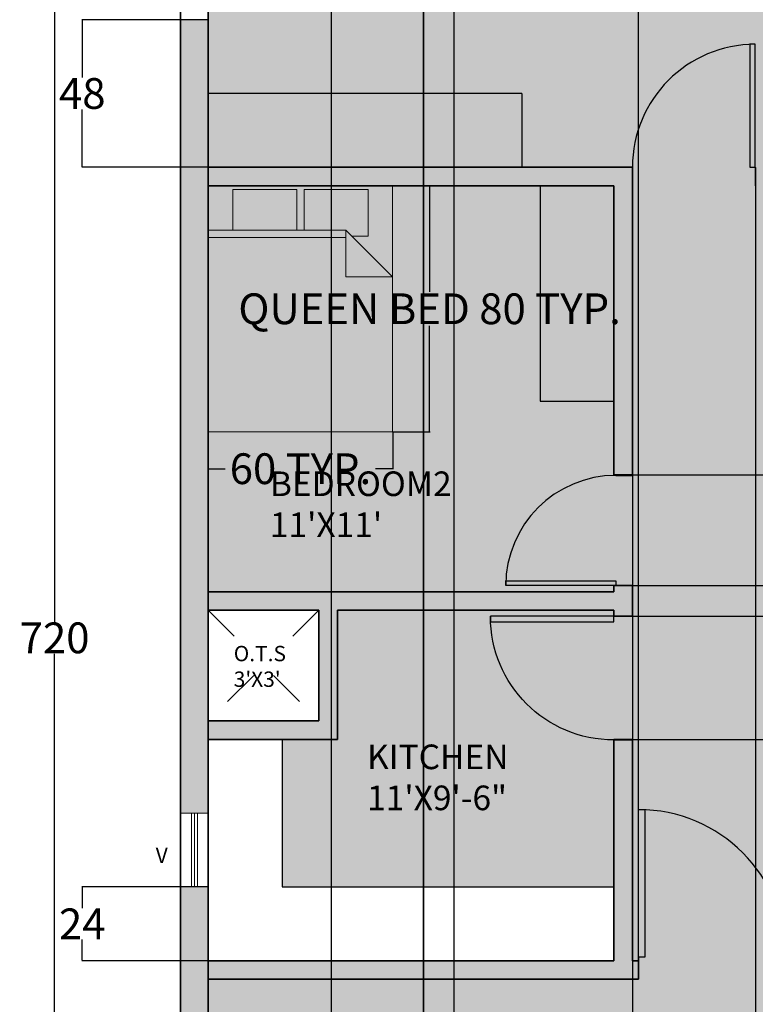
# Model space of a CAD drawing. Units: inches. Extents: x 286 to 756, y 360 to 1175.
# Tile 2 of 4: x 286 to 525, y 649 to 969. Entities that reach past the tile are written whole.
import ezdxf

# ---------------------------------------------------------------- set-up
doc = ezdxf.new("R2010")
doc.units = ezdxf.units.IN
doc.header["$MEASUREMENT"] = 0
doc.linetypes.add('ACAD_ISO03W100', pattern=[30, 12, -18])
for name, color, linetype, lineweight in [('A-ANNO-DIMS', 2, 'Continuous', 18), ('A-ANNO-TEXT', 7, 'Continuous', 18), ('A-AREA-IDEN', 7, 'Continuous', 18), ('A-FLOR-CASE', 8, 'Continuous', 25), ('A-FLOR-OPEN', 8, 'ACAD_ISO03W100', 13), ('A-GLAZ', 4, 'Continuous', 18), ('A-WALL', 7, 'Continuous', 35), ('DOOR', 6, 'Continuous', 25), ('FUR', 8, 'Continuous', 18)]:
    doc.layers.add(name, color=color, linetype=linetype, lineweight=lineweight)
for name, color, linetype, lineweight, true_color in [('A-FLOR-CASE-PATT', 30, 'Continuous', 13, 0xf8991e), ('A-FLOR-PATT', 9, 'Continuous', 13, 0xc7c8ca), ('A-WALL-PATT', 18, 'Continuous', 13, 0x000000)]:
    doc.layers.add(name, color=color, linetype=linetype, lineweight=lineweight, true_color=true_color)
doc.styles.get("Standard").update_dxf_attribs({"font": 'arial.ttf'})
doc.dimstyles.get("Standard").update_dxf_attribs({"dimtxt": 10, "dimasz": 0.18, "dimexe": 0.18, "dimexo": 0.0625, "dimgap": 0.09, "dimtad": 0, "dimtih": 1, "dimtoh": 1, "dimdec": 0, "dimzin": 0, "dimdsep": 46, "dimlunit": 3, "dimtxsty": 'Standard', "dimcen": 0.09, "dimadec": 0, "dimazin": 0, "dimtfac": 1, "dimtdec": 0, "dimtofl": 0, "dimtmove": 0, "dimatfit": 3, "dimfxl": 1, "dimtolj": 1, "dimtzin": 0, "dimarcsym": 0})

# ---------------------------------------------------------------- blocks, each defined once
blk = doc.blocks.new('*U7')
for p, q in [((0, 0), (0, -6)), ((-40, 0), (-40, -6))]:
    blk.add_line(p, q)
blk.add_lwpolyline([(0, 0), (0, 40), (-1.75, 40), (-1.75, 0)], close=True)
blk.add_arc((0, 0), 40, 90, 180)
blk = doc.blocks.new('Bed - Queen')
for p, q in [((0, -80.00003), (0, 0)), ((0, 0), (59.99999, 0)), ((59.99999, 0), (59.99999, -80.00003)), ((7.99999, -1.2), (28.79998, -1.2)), ((7.99999, -14.4), (7.99999, -1.2)), ((28.79998, -1.2), (28.79998, -14.4)), ((31.19999, -1.2), (51.99999, -1.2)), ((31.19999, -14.4), (31.19999, -1.2)), ((51.99999, -1.2), (51.99999, -16.4)), ((0, -14.4), (44.8, -14.4)), ((59.99999, -29.6), (44.8, -14.4)), ((44.8, -14.4), (44.8, -29.6)), ((44.8, -16.8), (0, -16.8)), ((51.99999, -16.4), (46.79936, -16.4)), ((44.8, -29.6), (59.99999, -29.6)), ((59.99999, -80.00003), (0, -80.00003))]:
    blk.add_line(p, q)
blk = doc.blocks.new('*U2')
for p, q in [((0, 0), (0, -6)), ((40, 0), (40, -6))]:
    blk.add_line(p, q)
blk.add_lwpolyline([(0, 0), (0, 40), (1.75, 40), (1.75, 0)], close=True)
blk.add_arc((0, 0), 40, 0, 90)
blk = doc.blocks.new('*U8')
for p, q in [((0, 0), (0, -6)), ((40, 0), (40, -6))]:
    blk.add_line(p, q)
blk.add_lwpolyline([(0, 0), (0, 40), (1.75, 40), (1.75, 0)], close=True)
blk.add_arc((0, 0), 40, 0, 90)
blk = doc.blocks.new('*D11')
at = {"layer": 'A-ANNO-DIMS', "color": 0, "lineweight": -2, "transparency": 16777216}
for p, q in [((406.93, 914.76), (419.05, 914.76)), ((418.87, 914.58), (418.87, 880.32)), ((418.87, 834.94), (418.87, 869.19)), ((406.93, 834.76), (419.05, 834.76))]:
    blk.add_line(p, q, dxfattribs=at)
at = {"layer": 'A-ANNO-DIMS', "color": 0, "transparency": 16777216}
for points in [[(418.84, 914.58), (418.9, 914.58), (418.87, 914.76)], [(418.84, 834.94), (418.9, 834.94), (418.87, 834.76)]]:
    blk.add_solid(points, dxfattribs=at)
at = {"layer": 'Defpoints', "color": 0, "transparency": 16777216}
for p in [(406.87, 914.76), (418.87, 914.76), (406.87, 834.76)]:
    blk.add_point(p, dxfattribs=at)
at = {"layer": 'A-ANNO-DIMS', "color": 0, "transparency": 16777216, "insert": (418.87, 874.76), "char_height": 10, "attachment_point": 5}
blk.add_mtext('\\A1;QUEEN BED 80 TYP.', dxfattribs=at)
blk = doc.blocks.new('*D12')
at = {"layer": 'A-ANNO-DIMS', "color": 0, "lineweight": -2, "transparency": 16777216}
for p, q in [((346.87, 834.69), (346.87, 822.58)), ((406.87, 834.69), (406.87, 822.58)), ((347.05, 822.76), (352.41, 822.76)), ((406.69, 822.76), (401.32, 822.76))]:
    blk.add_line(p, q, dxfattribs=at)
at = {"layer": 'A-ANNO-DIMS', "color": 0, "transparency": 16777216}
for points in [[(347.05, 822.79), (347.05, 822.73), (346.87, 822.76)], [(406.69, 822.79), (406.69, 822.73), (406.87, 822.76)]]:
    blk.add_solid(points, dxfattribs=at)
at = {"layer": 'Defpoints', "color": 0, "transparency": 16777216}
for p in [(346.87, 834.76), (406.87, 834.76), (406.87, 822.76)]:
    blk.add_point(p, dxfattribs=at)
at = {"layer": 'A-ANNO-DIMS', "color": 0, "transparency": 16777216, "insert": (376.87, 822.76), "char_height": 10, "attachment_point": 5}
blk.add_mtext('\\A1;60 TYP.', dxfattribs=at)
blk = doc.blocks.new('*D20')
at = {"layer": 'A-ANNO-DIMS', "color": 0, "lineweight": -2, "transparency": 16777216}
for p, q in [((346.8, 686.76), (305.69, 686.76)), ((305.87, 686.58), (305.87, 679.87)), ((305.87, 662.94), (305.87, 669.65)), ((346.8, 662.76), (305.69, 662.76))]:
    blk.add_line(p, q, dxfattribs=at)
at = {"layer": 'A-ANNO-DIMS', "color": 0, "transparency": 16777216}
for points in [[(305.84, 686.58), (305.9, 686.58), (305.87, 686.76)], [(305.84, 662.94), (305.9, 662.94), (305.87, 662.76)]]:
    blk.add_solid(points, dxfattribs=at)
at = {"layer": 'Defpoints', "color": 0, "transparency": 16777216}
for p in [(305.87, 686.76), (346.87, 686.76), (346.87, 662.76)]:
    blk.add_point(p, dxfattribs=at)
at = {"layer": 'A-ANNO-DIMS', "color": 0, "transparency": 16777216, "insert": (305.87, 674.76), "char_height": 10, "attachment_point": 5}
blk.add_mtext('\\A1;24', dxfattribs=at)
blk = doc.blocks.new('*D21')
at = {"layer": 'A-ANNO-DIMS', "color": 0, "lineweight": -2, "transparency": 16777216}
for p, q in [((346.8, 968.76), (305.69, 968.76)), ((305.87, 968.58), (305.87, 949.95)), ((305.87, 920.94), (305.87, 939.56)), ((346.8, 920.76), (305.69, 920.76))]:
    blk.add_line(p, q, dxfattribs=at)
at = {"layer": 'A-ANNO-DIMS', "color": 0, "transparency": 16777216}
for points in [[(305.84, 968.58), (305.9, 968.58), (305.87, 968.76)], [(305.84, 920.94), (305.9, 920.94), (305.87, 920.76)]]:
    blk.add_solid(points, dxfattribs=at)
at = {"layer": 'Defpoints', "color": 0, "transparency": 16777216}
for p in [(305.87, 968.76), (346.87, 968.76), (346.87, 920.76)]:
    blk.add_point(p, dxfattribs=at)
at = {"layer": 'A-ANNO-DIMS', "color": 0, "transparency": 16777216, "insert": (305.87, 944.76), "char_height": 10, "attachment_point": 5}
blk.add_mtext('\\A1;48', dxfattribs=at)
blk = doc.blocks.new('*D22')
at = {"layer": 'A-ANNO-DIMS', "color": 0, "lineweight": -2, "transparency": 16777216}
for p, q in [((337.8, 1127.76), (296.69, 1127.76)), ((296.87, 1127.58), (296.87, 772.95)), ((296.87, 407.94), (296.87, 762.56)), ((337.8, 407.76), (296.69, 407.76))]:
    blk.add_line(p, q, dxfattribs=at)
at = {"layer": 'A-ANNO-DIMS', "color": 0, "transparency": 16777216}
for points in [[(296.84, 1127.58), (296.9, 1127.58), (296.87, 1127.76)], [(296.84, 407.94), (296.9, 407.94), (296.87, 407.76)]]:
    blk.add_solid(points, dxfattribs=at)
at = {"layer": 'Defpoints', "color": 0, "transparency": 16777216}
for p in [(296.87, 1127.76), (337.87, 1127.76), (337.87, 407.76)]:
    blk.add_point(p, dxfattribs=at)
at = {"layer": 'A-ANNO-DIMS', "color": 0, "transparency": 16777216, "insert": (296.87, 767.76), "char_height": 10, "attachment_point": 5}
blk.add_mtext('\\A1;720', dxfattribs=at)
blk = doc.blocks.new('*D26')
at = {"layer": 'A-ANNO-DIMS', "color": 0, "lineweight": -2, "transparency": 16777216}
for p, q in [((346.87, 656.82), (346.87, 1168.94)), ((347.05, 1168.76), (406.22, 1168.76)), ((486.69, 1168.76), (427.51, 1168.76)), ((486.87, 656.82), (486.87, 1168.94))]:
    blk.add_line(p, q, dxfattribs=at)
at = {"layer": 'A-ANNO-DIMS', "color": 0, "transparency": 16777216}
for points in [[(347.05, 1168.79), (347.05, 1168.73), (346.87, 1168.76)], [(486.69, 1168.79), (486.69, 1168.73), (486.87, 1168.76)]]:
    blk.add_solid(points, dxfattribs=at)
at = {"layer": 'Defpoints', "color": 0, "transparency": 16777216}
for p in [(486.87, 1168.76), (346.87, 656.76), (486.87, 656.76)]:
    blk.add_point(p, dxfattribs=at)
at = {"layer": 'A-ANNO-DIMS', "color": 0, "transparency": 16777216, "insert": (416.87, 1168.76), "char_height": 10, "attachment_point": 5}
blk.add_mtext('\\A1;140', dxfattribs=at)
blk = doc.blocks.new('*D27')
at = {"layer": 'A-ANNO-DIMS', "color": 0, "lineweight": -2, "transparency": 16777216}
for p, q in [((486.87, 656.82), (486.87, 1168.94)), ((487.05, 1168.76), (503.4, 1168.76)), ((534.69, 1168.76), (518.33, 1168.76)), ((534.87, 656.82), (534.87, 1168.94))]:
    blk.add_line(p, q, dxfattribs=at)
at = {"layer": 'A-ANNO-DIMS', "color": 0, "transparency": 16777216}
for points in [[(487.05, 1168.79), (487.05, 1168.73), (486.87, 1168.76)], [(534.69, 1168.79), (534.69, 1168.73), (534.87, 1168.76)]]:
    blk.add_solid(points, dxfattribs=at)
at = {"layer": 'Defpoints', "color": 0, "transparency": 16777216}
for p in [(534.87, 1168.76), (486.87, 656.76), (534.87, 656.76)]:
    blk.add_point(p, dxfattribs=at)
at = {"layer": 'A-ANNO-DIMS', "color": 0, "transparency": 16777216, "insert": (510.87, 1168.76), "char_height": 10, "attachment_point": 5}
blk.add_mtext('\\A1;48', dxfattribs=at)
blk = doc.blocks.new('*D33')
at = {"layer": 'A-ANNO-DIMS', "color": 0, "lineweight": -2, "transparency": 16777216}
for p, q in [((416.87, 452.82), (416.87, 1168.94)), ((417.05, 1168.76), (426.69, 1168.76)), ((426.87, 452.82), (426.87, 1168.94)), ((426.87, 1168.76), (427.05, 1168.76))]:
    blk.add_line(p, q, dxfattribs=at)
at = {"layer": 'A-ANNO-DIMS', "color": 0, "transparency": 16777216}
for points in [[(417.05, 1168.79), (417.05, 1168.73), (416.87, 1168.76)], [(426.69, 1168.79), (426.69, 1168.73), (426.87, 1168.76)]]:
    blk.add_solid(points, dxfattribs=at)
at = {"layer": 'Defpoints', "color": 0, "transparency": 16777216}
for p in [(426.87, 1168.76), (416.87, 452.76), (426.87, 452.76)]:
    blk.add_point(p, dxfattribs=at)
at = {"layer": 'A-ANNO-DIMS', "color": 0, "transparency": 16777216, "insert": (433.81, 1168.76), "char_height": 10, "attachment_point": 5}
blk.add_mtext('\\A1;10', dxfattribs=at)
blk = doc.blocks.new('*D34')
at = {"layer": 'A-ANNO-DIMS', "color": 0, "lineweight": -2, "transparency": 16777216}
for p, q in [((346.87, 1064.69), (346.87, 366.58)), ((386.87, 1064.69), (386.87, 366.58)), ((347.05, 366.76), (359.43, 366.76)), ((386.69, 366.76), (374.3, 366.76))]:
    blk.add_line(p, q, dxfattribs=at)
at = {"layer": 'A-ANNO-DIMS', "color": 0, "transparency": 16777216}
for points in [[(347.05, 366.79), (347.05, 366.73), (346.87, 366.76)], [(386.69, 366.79), (386.69, 366.73), (386.87, 366.76)]]:
    blk.add_solid(points, dxfattribs=at)
at = {"layer": 'Defpoints', "color": 0, "transparency": 16777216}
for p in [(346.87, 1064.76), (386.87, 1064.76), (386.87, 366.76)]:
    blk.add_point(p, dxfattribs=at)
at = {"layer": 'A-ANNO-DIMS', "color": 0, "transparency": 16777216, "insert": (366.87, 366.76), "char_height": 10, "attachment_point": 5}
blk.add_mtext('\\A1;40', dxfattribs=at)
blk = doc.blocks.new('*D35')
at = {"layer": 'A-ANNO-DIMS', "color": 0, "lineweight": -2, "transparency": 16777216}
for p, q in [((386.87, 1064.69), (386.87, 366.58)), ((416.87, 1064.69), (416.87, 366.58)), ((387.05, 366.76), (394.63, 366.76)), ((416.69, 366.76), (409.1, 366.76))]:
    blk.add_line(p, q, dxfattribs=at)
at = {"layer": 'A-ANNO-DIMS', "color": 0, "transparency": 16777216}
for points in [[(387.05, 366.79), (387.05, 366.73), (386.87, 366.76)], [(416.69, 366.79), (416.69, 366.73), (416.87, 366.76)]]:
    blk.add_solid(points, dxfattribs=at)
at = {"layer": 'Defpoints', "color": 0, "transparency": 16777216}
for p in [(386.87, 1064.76), (416.87, 1064.76), (416.87, 366.76)]:
    blk.add_point(p, dxfattribs=at)
at = {"layer": 'A-ANNO-DIMS', "color": 0, "transparency": 16777216, "insert": (401.87, 366.76), "char_height": 10, "attachment_point": 5}
blk.add_mtext('\\A1;30', dxfattribs=at)
blk = doc.blocks.new('*D37')
at = {"layer": 'A-ANNO-DIMS', "color": 0, "lineweight": -2, "transparency": 16777216}
for p, q in [((478.93, 774.76), (739.05, 774.76)), ((738.87, 774.58), (738.87, 759.95)), ((738.87, 734.94), (738.87, 749.56)), ((478.93, 734.76), (739.05, 734.76))]:
    blk.add_line(p, q, dxfattribs=at)
at = {"layer": 'A-ANNO-DIMS', "color": 0, "transparency": 16777216}
for points in [[(738.84, 774.58), (738.9, 774.58), (738.87, 774.76)], [(738.84, 734.94), (738.9, 734.94), (738.87, 734.76)]]:
    blk.add_solid(points, dxfattribs=at)
at = {"layer": 'Defpoints', "color": 0, "transparency": 16777216}
for p in [(478.87, 774.76), (738.87, 774.76), (478.87, 734.76)]:
    blk.add_point(p, dxfattribs=at)
at = {"layer": 'A-ANNO-DIMS', "color": 0, "transparency": 16777216, "insert": (738.87, 754.76), "char_height": 10, "attachment_point": 5}
blk.add_mtext('\\A1;40', dxfattribs=at)
blk = doc.blocks.new('*D38')
at = {"layer": 'A-ANNO-DIMS', "color": 0, "lineweight": -2, "transparency": 16777216}
for p, q in [((478.93, 820.76), (739.05, 820.76)), ((738.87, 820.58), (738.87, 807.95)), ((738.87, 784.94), (738.87, 797.56)), ((478.93, 784.76), (739.05, 784.76))]:
    blk.add_line(p, q, dxfattribs=at)
at = {"layer": 'A-ANNO-DIMS', "color": 0, "transparency": 16777216}
for points in [[(738.84, 820.58), (738.9, 820.58), (738.87, 820.76)], [(738.84, 784.94), (738.9, 784.94), (738.87, 784.76)]]:
    blk.add_solid(points, dxfattribs=at)
at = {"layer": 'Defpoints', "color": 0, "transparency": 16777216}
for p in [(478.87, 820.76), (738.87, 820.76), (478.87, 784.76)]:
    blk.add_point(p, dxfattribs=at)
at = {"layer": 'A-ANNO-DIMS', "color": 0, "transparency": 16777216, "insert": (738.87, 802.76), "char_height": 10, "attachment_point": 5}
blk.add_mtext('\\A1;36', dxfattribs=at)
blk = doc.blocks.new('*D39')
at = {"layer": 'A-ANNO-DIMS', "color": 0, "lineweight": -2, "transparency": 16777216}
for p, q in [((484.87, 920.69), (484.87, 366.58)), ((524.87, 920.69), (524.87, 366.58)), ((485.05, 366.76), (497.43, 366.76)), ((524.69, 366.76), (512.3, 366.76))]:
    blk.add_line(p, q, dxfattribs=at)
at = {"layer": 'A-ANNO-DIMS', "color": 0, "transparency": 16777216}
for points in [[(485.05, 366.79), (485.05, 366.73), (484.87, 366.76)], [(524.69, 366.79), (524.69, 366.73), (524.87, 366.76)]]:
    blk.add_solid(points, dxfattribs=at)
at = {"layer": 'Defpoints', "color": 0, "transparency": 16777216}
for p in [(484.87, 920.76), (524.87, 920.76), (524.87, 366.76)]:
    blk.add_point(p, dxfattribs=at)
at = {"layer": 'A-ANNO-DIMS', "color": 0, "transparency": 16777216, "insert": (504.87, 366.76), "char_height": 10, "attachment_point": 5}
blk.add_mtext('\\A1;40', dxfattribs=at)

msp = doc.modelspace()

# ---------------------------------------------------------------- hatches: boundary and pattern name
at = {"layer": 'A-FLOR-CASE-PATT'}
h = msp.add_hatch(color=256, dxfattribs=at)
h.dxf.hatch_style = 1
h.paths.add_polyline_path([(448.865, 944.756), (346.865, 944.756), (346.865, 920.756), (448.865, 920.756)])
h.paths.add_polyline_path([(478.865, 914.756), (454.865, 914.756), (454.865, 844.756), (478.865, 844.756)])
h.paths.add_polyline_path([(688.865, 944.756), (586.865, 944.756), (586.865, 920.756), (688.865, 920.756)])
at = {"layer": 'A-FLOR-PATT'}
h = msp.add_hatch(color=256, dxfattribs=at)
h.dxf.hatch_style = 1
h.paths.add_polyline_path([(526.865, 1064.756), (386.892, 1064.756), (346.865, 1064.756), (346.865, 944.756), (448.865, 944.756), (448.865, 920.756), (484.865, 920.756), (484.865, 914.756), (524.865, 914.756), (524.865, 920.756), (526.865, 920.756)])
h.paths.add_polyline_path([(418.865, 1118.756), (346.865, 1118.756), (346.865, 1070.756), (386.865, 1070.756), (386.865, 1064.756), (386.892, 1064.756), (416.865, 1064.756), (416.865, 1070.756), (418.865, 1070.756)])
h.paths.add_polyline_path([(526.865, 1118.756), (424.865, 1118.756), (424.865, 1070.756), (494.865, 1070.756), (494.865, 1064.756), (524.865, 1064.756), (524.865, 1070.756), (526.865, 1070.756)])
h.paths.add_polyline_path([(610.865, 1118.756), (532.865, 1118.756), (532.865, 1070.756), (534.865, 1070.756), (534.865, 1064.756), (564.865, 1064.756), (564.865, 1070.756), (610.865, 1070.756)])
h.paths.add_polyline_path([(688.865, 1118.756), (616.865, 1118.756), (616.865, 1070.756), (618.865, 1070.756), (618.865, 1064.756), (648.865, 1064.756), (648.865, 1070.756), (688.865, 1070.756)])
h.paths.add_polyline_path([(688.865, 1064.756), (648.865, 1064.756), (618.865, 1064.756), (532.865, 1064.756), (532.865, 920.756), (534.865, 920.756), (534.865, 914.756), (570.865, 914.756), (570.865, 920.756), (586.865, 920.756), (586.865, 944.756), (688.865, 944.756)])
h.paths.add_polyline_path([(484.865, 820.756), (478.865, 820.756), (478.865, 844.756), (454.865, 844.756), (454.865, 914.756), (346.865, 914.756), (346.865, 782.756), (478.865, 782.756), (478.865, 784.756), (484.865, 784.756)])
h.paths.add_polyline_path([(688.865, 914.756), (570.865, 914.756), (534.865, 914.756), (484.865, 914.756), (484.865, 820.756), (484.865, 784.756), (484.865, 734.577), (484.865, 662.756), (486.865, 662.756), (486.865, 656.756), (534.865, 656.756), (534.865, 662.756), (688.865, 662.756)])
h.paths.add_polyline_path([(478.865, 734.756), (484.865, 734.756), (484.865, 774.756), (478.865, 774.756), (478.865, 776.756), (388.865, 776.756), (388.865, 734.756), (370.865, 734.756), (370.865, 686.756), (478.865, 686.756)])
h.paths.add_polyline_path([(688.865, 656.756), (534.865, 656.756), (486.865, 656.756), (484.865, 656.756), (346.865, 656.756), (346.865, 536.756), (388.865, 536.756), (388.865, 530.756), (388.865, 506.756), (388.865, 488.756), (388.865, 464.756), (388.865, 452.756), (466.865, 452.756), (466.865, 416.756), (496.865, 416.756), (544.865, 416.756), (580.865, 416.756), (688.865, 416.756)])
h.paths.add_polyline_path([(388.865, 530.756), (346.865, 530.756), (346.865, 494.756), (382.865, 494.756), (382.865, 506.756), (388.865, 506.756)], flags=17)
h.paths.add_polyline_path([(382.865, 464.756), (388.865, 464.756), (388.865, 488.756), (346.865, 488.756), (346.865, 452.756), (382.865, 452.756)], flags=17)
at = {"layer": 'A-WALL-PATT'}
h = msp.add_hatch(color=256, dxfattribs=at)
h.dxf.hatch_style = 1
h.paths.add_polyline_path([(496.865, 416.756), (346.865, 416.756), (346.865, 656.756), (484.865, 656.756), (486.865, 656.756), (486.865, 662.756), (484.865, 662.756), (484.865, 734.577), (478.865, 734.577), (478.865, 662.756), (346.865, 662.756), (346.865, 686.756), (337.865, 686.756), (337.865, 407.756), (496.865, 407.756)])
h.paths.add_polyline_path([(484.865, 784.756), (478.865, 784.756), (478.865, 782.756), (346.865, 782.756), (346.865, 914.756), (406.865, 914.756), (478.865, 914.756), (478.865, 820.756), (484.865, 820.756), (484.865, 920.756), (346.865, 920.756), (346.865, 968.756), (337.865, 968.756), (337.865, 710.756), (346.865, 710.756), (346.865, 734.756), (388.865, 734.756), (388.865, 776.756), (478.865, 776.756), (478.865, 774.756), (484.865, 774.756)])
h.paths.add_polyline_path([(382.865, 776.756), (382.865, 740.756), (346.865, 740.756), (346.865, 776.756)], flags=16)
h.paths.add_polyline_path([(386.865, 1070.756), (346.865, 1070.756), (346.865, 1118.756), (418.865, 1118.756), (418.865, 1106.756), (424.865, 1106.756), (424.865, 1118.756), (526.865, 1118.756), (526.865, 1070.756), (532.865, 1070.756), (532.865, 1118.756), (610.865, 1118.756), (610.865, 1106.756), (616.865, 1106.756), (616.865, 1118.756), (688.865, 1118.756), (688.865, 1016.756), (697.865, 1016.756), (697.865, 1127.756), (337.865, 1127.756), (337.865, 1016.756), (346.865, 1016.756), (346.865, 1030.663), (346.865, 1064.756), (386.865, 1064.756)])
h.paths.add_polyline_path([(494.822, 1069.262, -0.0124335), (494.859, 1070.756), (424.865, 1070.756), (424.865, 1082.756), (418.865, 1082.756), (418.865, 1070.756), (416.865, 1070.756), (416.865, 1069.252), (416.865, 1064.756), (494.822, 1064.756)], flags=17)
h.paths.add_polyline_path([(618.865, 1069.261), (618.865, 1070.756), (616.865, 1070.756), (616.865, 1082.756), (610.865, 1082.756), (610.865, 1070.756), (564.872, 1070.756, -0.0124335), (564.909, 1069.262), (564.909, 1064.756), (618.865, 1064.756)], flags=17)
h.paths.add_polyline_path([(688.865, 1070.756), (648.865, 1070.756), (648.865, 1070.756, -0.0124418), (648.902, 1069.261), (648.902, 1064.756), (688.865, 1064.756)], flags=17)
h.paths.add_polyline_path([(697.865, 968.756), (688.865, 968.756), (688.865, 920.756), (570.865, 920.756), (570.865, 914.756), (688.865, 914.756), (688.865, 873.949), (697.865, 873.949)])
h.paths.add_polyline_path([(697.865, 825.949), (688.865, 825.949), (688.865, 756.879), (697.865, 756.879)])
h.paths.add_polyline_path([(532.865, 1064.756), (526.865, 1064.756), (526.865, 920.756), (524.865, 920.756), (524.865, 914.756), (534.865, 914.756), (534.865, 920.756), (532.865, 920.756)])

# ---------------------------------------------------------------- linework, layer by layer
at = {"layer": 'A-FLOR-CASE'}
for p, q in [((448.865, 944.756), (346.865, 944.756)), ((448.865, 944.756), (448.865, 920.756)), ((454.865, 914.756), (454.865, 844.756)), ((454.865, 844.756), (478.865, 844.756)), ((370.865, 734.756), (370.865, 686.756)), ((370.865, 686.756), (478.865, 686.756))]:
    msp.add_line(p, q, dxfattribs=at)
at = {"layer": 'A-FLOR-OPEN'}
for p, q in [((382.865, 776.756), (346.865, 740.756)), ((346.865, 776.756), (382.865, 740.756))]:
    msp.add_line(p, q, dxfattribs=at)
at = {"layer": 'A-GLAZ'}
for p, q in [((346.865, 710.756), (337.865, 710.756)), ((341.365, 710.756), (341.365, 686.756)), ((342.365, 710.756), (342.365, 686.756)), ((343.365, 710.756), (343.365, 686.756)), ((346.865, 686.756), (337.865, 686.756))]:
    msp.add_line(p, q, dxfattribs=at)
at = {"layer": 'A-WALL'}
for p, q in [((337.865, 1127.756), (337.865, 407.756)), ((346.865, 1064.756), (346.865, 920.756)), ((346.865, 920.756), (346.865, 1064.756)), ((484.865, 920.756), (346.865, 920.756)), ((484.865, 920.756), (484.865, 820.756)), ((478.865, 914.756), (346.865, 914.756)), ((346.865, 914.756), (346.865, 782.756)), ((478.865, 914.756), (478.865, 820.756)), ((484.865, 820.756), (478.865, 820.756)), ((478.865, 782.756), (478.865, 784.756)), ((478.865, 784.756), (484.865, 784.756)), ((484.865, 784.756), (484.865, 782.756)), ((478.865, 782.756), (346.865, 782.756)), ((484.865, 782.756), (484.865, 776.756)), ((382.865, 776.756), (346.865, 776.756)), ((346.865, 776.756), (346.865, 740.756)), ((382.865, 776.756), (382.865, 740.756)), ((478.865, 776.756), (388.865, 776.756)), ((388.865, 776.756), (388.865, 734.756)), ((478.865, 774.756), (478.865, 776.756)), ((484.865, 776.756), (484.865, 774.756)), ((484.865, 774.756), (478.865, 774.756)), ((382.865, 740.756), (346.865, 740.756)), ((388.865, 734.756), (346.865, 734.756)), ((346.865, 734.756), (346.865, 662.756)), ((346.865, 662.756), (346.865, 734.756)), ((478.865, 734.756), (478.865, 662.756)), ((484.865, 734.756), (478.865, 734.756)), ((484.865, 734.756), (484.865, 662.756)), ((346.865, 662.756), (478.865, 662.756)), ((486.865, 662.756), (484.865, 662.756)), ((486.865, 656.756), (486.865, 662.756)), ((346.865, 656.756), (484.865, 656.756)), ((346.865, 656.756), (346.865, 416.756)), ((484.865, 656.756), (486.865, 656.756))]:
    msp.add_line(p, q, dxfattribs=at)

# ---------------------------------------------------------------- block references
at = {"layer": 'DOOR'}
msp.add_blockref('*U7', (524.865, 920.756), dxfattribs=at)
at = {"layer": 'DOOR', "rotation": 90}
for p, xscale, yscale, zscale in [((479.491, 784.756), 0.8957208258830688, 0.8957208258830688, 0.8957208258830688), ((478.838, 774.756), -1.004475396251834, 1.004475396251834, 1.004475396251834)]:
    msp.add_blockref('*U2', p, dxfattribs=dict(at, xscale=xscale, yscale=yscale, zscale=zscale))
at = {"layer": 'DOOR', "xscale": 1.198937203557198, "yscale": 1.198937203557198, "zscale": 1.198937203557198}
msp.add_blockref('*U8', (486.865, 663.949), dxfattribs=at)
at = {"layer": 'FUR'}
msp.add_blockref('Bed - Queen', (346.865, 914.756), dxfattribs=at)

# ---------------------------------------------------------------- texts
at = {"layer": 'A-ANNO-TEXT', "insert": (329.766, 699.546), "char_height": 5, "attachment_point": 1}
msp.add_mtext_dynamic_manual_height_columns('V', width=36.25002, gutter_width=1, heights=[0], dxfattribs=at)
at = {"layer": 'A-AREA-IDEN', "attachment_point": 1}
for s, insert, char_height in [("BEDROOM2\\P11'X11'", (366.91, 821.865), 8), ("O.T.S\\P3'X3'", (355.15, 765.152), 5), ('KITCHEN\\P11\'X9\'-6"', (398.55, 733.066), 8)]:
    msp.add_mtext_dynamic_manual_height_columns(s, width=59.48304, gutter_width=1, heights=[0], dxfattribs=dict(at, insert=insert, char_height=char_height))

# ---------------------------------------------------------------- dimensions: what is measured, and where the dimension line sits
at = {"layer": 'A-ANNO-DIMS'}
for base, p1, p2, picture, middle in [((486.865, 1168.756), (346.865, 656.756), (486.865, 656.756), '*D26', (416.865, 1168.756)), ((426.865, 1168.756), (416.865, 452.756), (426.865, 452.756), '*D33', (433.81, 1168.756)), ((534.865, 1168.756), (486.865, 656.756), (534.865, 656.756), '*D27', (510.865, 1168.756)), ((386.865, 366.756), (346.865, 1064.756), (386.865, 1064.756), '*D34', (366.865, 366.756)), ((416.865, 366.756), (386.865, 1064.756), (416.865, 1064.756), '*D35', (401.865, 366.756)), ((524.865, 366.756), (484.865, 920.756), (524.865, 920.756), '*D39', (504.865, 366.756))]:
    dim = msp.add_linear_dim(base=base, p1=p1, p2=p2, dimstyle='Standard', override={"dimdec": 0, "dimlfac": 1, "dimrnd": 0, "dimzin": 0, "dimdsep": 46, "dimlunit": 2}, dxfattribs=at)
    dim.commit()
    dim.dimension.update_dxf_attribs({"geometry": picture, "text_midpoint": middle})
for base, p1, p2, picture, middle in [((296.865, 1127.756), (337.865, 407.756), (337.865, 1127.756), '*D22', (296.865, 767.756)), ((305.865, 968.756), (346.865, 920.756), (346.865, 968.756), '*D21', (305.865, 944.756)), ((738.865, 820.756), (478.865, 784.756), (478.865, 820.756), '*D38', (738.865, 802.756)), ((738.865, 774.756), (478.865, 734.756), (478.865, 774.756), '*D37', (738.865, 754.756)), ((305.865, 686.756), (346.865, 662.756), (346.865, 686.756), '*D20', (305.865, 674.756))]:
    dim = msp.add_linear_dim(base=base, p1=p1, p2=p2, angle=90, dimstyle='Standard', override={"dimdec": 0, "dimlfac": 1, "dimrnd": 0, "dimzin": 0, "dimdsep": 46, "dimlunit": 2}, dxfattribs=at)
    dim.commit()
    dim.dimension.update_dxf_attribs({"geometry": picture, "text_midpoint": middle})
dim = msp.add_linear_dim(base=(418.865, 914.756), p1=(406.865, 834.756), p2=(406.865, 914.756), angle=90, text='QUEEN BED <> TYP.', dimstyle='Standard', override={"dimdec": 0, "dimlfac": 1, "dimrnd": 0, "dimzin": 0, "dimdsep": 46, "dimlunit": 2}, dxfattribs=at)
dim.commit()
dim.dimension.update_dxf_attribs({"geometry": '*D11', "text_midpoint": (418.865, 874.756)})
dim = msp.add_linear_dim(base=(406.865, 822.756), p1=(346.865, 834.756), p2=(406.865, 834.756), text='<> TYP.', dimstyle='Standard', override={"dimdec": 0, "dimlfac": 1, "dimrnd": 0, "dimzin": 0, "dimdsep": 46, "dimlunit": 2}, dxfattribs=at)
dim.commit()
dim.dimension.update_dxf_attribs({"geometry": '*D12', "text_midpoint": (376.865, 822.756)})

doc.saveas('drawing.dxf')
